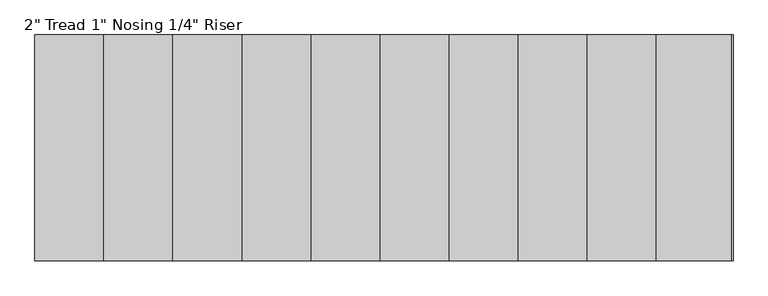
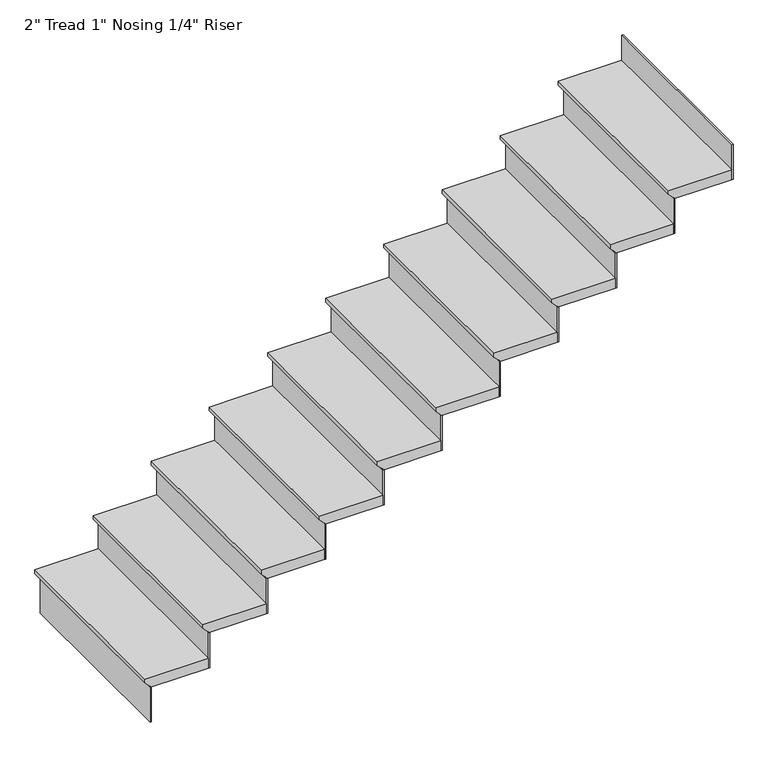
"""IFC4 building model written with IfcOpenShell, lengths in millimetres: stair flight geometry."""

from ifc_helpers import new_model, si_unit, frame, origin, place, context, project, spatial, polyline, outline, extrude, source, transform, mapped, element, save


def stair_flight_87f1d909(model_context):
    return source(origin(), model_context, "Body", "SweptSolid", [
        extrude(outline(polyline([(8432.8, -7947.6763529), (8432.8, -8252.4763529), (8413.75, -8252.4763529), (8388.35, -8227.0763529), (8382.0, -8227.0763529), (8382.0, -7947.6763529), (8432.8, -7947.6763529)])), frame((0.0, -3490.0338022, 0.0), z_axis=(0.0, 1.0, 0.0), x_axis=(0.0, 0.0, 1.0)), (0.0, 0.0, 1.0), 914.4),
        extrude(outline(polyline([(-8220.7263529, -3490.0338022), (-8227.0763529, -3490.0338022), (-8227.0763529, -2575.6338022), (-8220.7263529, -2575.6338022), (-8220.7263529, -3490.0338022)])), frame((0.0, 0.0, 8204.2), z_axis=(0.0, 0.0, 1.0), x_axis=(1.0, 0.0, 0.0)), (0.0, 0.0, 1.0), 177.8),
        extrude(outline(polyline([(-7941.3263529, -3490.0338022), (-7947.6763529, -3490.0338022), (-7947.6763529, -2575.6338022), (-7941.3263529, -2575.6338022), (-7941.3263529, -3490.0338022)])), frame((0.0, 0.0, 8382.0), z_axis=(0.0, 0.0, 1.0), x_axis=(1.0, 0.0, 0.0)), (0.0, 0.0, 1.0), 177.8),
        extrude(outline(polyline([(8610.6, -7668.2763529), (8610.6, -7973.0763529), (8591.55, -7973.0763529), (8566.15, -7947.6763529), (8559.8, -7947.6763529), (8559.8, -7668.2763529), (8610.6, -7668.2763529)])), frame((0.0, -3490.0338022, 0.0), z_axis=(0.0, 1.0, 0.0), x_axis=(0.0, 0.0, 1.0)), (0.0, 0.0, 1.0), 914.4),
        extrude(outline(polyline([(-7661.9263529, -3490.0338022), (-7668.2763529, -3490.0338022), (-7668.2763529, -2575.6338022), (-7661.9263529, -2575.6338022), (-7661.9263529, -3490.0338022)])), frame((0.0, 0.0, 8559.8), z_axis=(0.0, 0.0, 1.0), x_axis=(1.0, 0.0, 0.0)), (0.0, 0.0, 1.0), 177.8),
        extrude(outline(polyline([(8788.4, -7388.8763529), (8788.4, -7693.6763529), (8769.35, -7693.6763529), (8743.95, -7668.2763529), (8737.6, -7668.2763529), (8737.6, -7388.8763529), (8788.4, -7388.8763529)])), frame((0.0, -3490.0338022, 0.0), z_axis=(0.0, 1.0, 0.0), x_axis=(0.0, 0.0, 1.0)), (0.0, 0.0, 1.0), 914.4),
        extrude(outline(polyline([(-7382.5263529, -3490.0338022), (-7388.8763529, -3490.0338022), (-7388.8763529, -2575.6338022), (-7382.5263529, -2575.6338022), (-7382.5263529, -3490.0338022)])), frame((0.0, 0.0, 8737.6), z_axis=(0.0, 0.0, 1.0), x_axis=(1.0, 0.0, 0.0)), (0.0, 0.0, 1.0), 177.8),
        extrude(outline(polyline([(8966.2, -7109.4763529), (8966.2, -7414.2763529), (8947.15, -7414.2763529), (8921.75, -7388.8763529), (8915.4, -7388.8763529), (8915.4, -7109.4763529), (8966.2, -7109.4763529)])), frame((0.0, -3490.0338022, 0.0), z_axis=(0.0, 1.0, 0.0), x_axis=(0.0, 0.0, 1.0)), (0.0, 0.0, 1.0), 914.4),
        extrude(outline(polyline([(-7103.1263529, -3490.0338022), (-7109.4763529, -3490.0338022), (-7109.4763529, -2575.6338022), (-7103.1263529, -2575.6338022), (-7103.1263529, -3490.0338022)])), frame((0.0, 0.0, 8915.4), z_axis=(0.0, 0.0, 1.0), x_axis=(1.0, 0.0, 0.0)), (0.0, 0.0, 1.0), 177.8),
        extrude(outline(polyline([(9144.0, -6830.0763529), (9144.0, -7134.8763529), (9124.95, -7134.8763529), (9099.55, -7109.4763529), (9093.2, -7109.4763529), (9093.2, -6830.0763529), (9144.0, -6830.0763529)])), frame((0.0, -3490.0338022, 0.0), z_axis=(0.0, 1.0, 0.0), x_axis=(0.0, 0.0, 1.0)), (0.0, 0.0, 1.0), 914.4),
        extrude(outline(polyline([(-6823.7263529, -3490.0338022), (-6830.0763529, -3490.0338022), (-6830.0763529, -2575.6338022), (-6823.7263529, -2575.6338022), (-6823.7263529, -3490.0338022)])), frame((0.0, 0.0, 9093.2), z_axis=(0.0, 0.0, 1.0), x_axis=(1.0, 0.0, 0.0)), (0.0, 0.0, 1.0), 177.8),
        extrude(outline(polyline([(9321.8, -6550.6763529), (9321.8, -6855.4763529), (9302.75, -6855.4763529), (9277.35, -6830.0763529), (9271.0, -6830.0763529), (9271.0, -6550.6763529), (9321.8, -6550.6763529)])), frame((0.0, -3490.0338022, 0.0), z_axis=(0.0, 1.0, 0.0), x_axis=(0.0, 0.0, 1.0)), (0.0, 0.0, 1.0), 914.4),
        extrude(outline(polyline([(-6544.3263529, -3490.0338022), (-6550.6763529, -3490.0338022), (-6550.6763529, -2575.6338022), (-6544.3263529, -2575.6338022), (-6544.3263529, -3490.0338022)])), frame((0.0, 0.0, 9271.0), z_axis=(0.0, 0.0, 1.0), x_axis=(1.0, 0.0, 0.0)), (0.0, 0.0, 1.0), 177.8),
        extrude(outline(polyline([(9499.6, -6271.2763529), (9499.6, -6576.0763529), (9480.55, -6576.0763529), (9455.15, -6550.6763529), (9448.8, -6550.6763529), (9448.8, -6271.2763529), (9499.6, -6271.2763529)])), frame((0.0, -3490.0338022, 0.0), z_axis=(0.0, 1.0, 0.0), x_axis=(0.0, 0.0, 1.0)), (0.0, 0.0, 1.0), 914.4),
        extrude(outline(polyline([(-6264.9263529, -3490.0338022), (-6271.2763529, -3490.0338022), (-6271.2763529, -2575.6338022), (-6264.9263529, -2575.6338022), (-6264.9263529, -3490.0338022)])), frame((0.0, 0.0, 9448.8), z_axis=(0.0, 0.0, 1.0), x_axis=(1.0, 0.0, 0.0)), (0.0, 0.0, 1.0), 177.8),
        extrude(outline(polyline([(9677.4, -5991.8763529), (9677.4, -6296.6763529), (9658.35, -6296.6763529), (9632.95, -6271.2763529), (9626.6, -6271.2763529), (9626.6, -5991.8763529), (9677.4, -5991.8763529)])), frame((0.0, -3490.0338022, 0.0), z_axis=(0.0, 1.0, 0.0), x_axis=(0.0, 0.0, 1.0)), (0.0, 0.0, 1.0), 914.4),
        extrude(outline(polyline([(-5985.5263529, -3490.0338022), (-5991.8763529, -3490.0338022), (-5991.8763529, -2575.6338022), (-5985.5263529, -2575.6338022), (-5985.5263529, -3490.0338022)])), frame((0.0, 0.0, 9626.6), z_axis=(0.0, 0.0, 1.0), x_axis=(1.0, 0.0, 0.0)), (0.0, 0.0, 1.0), 177.8),
        extrude(outline(polyline([(9855.2, -5712.4763529), (9855.2, -6017.2763529), (9836.15, -6017.2763529), (9810.75, -5991.8763529), (9804.4, -5991.8763529), (9804.4, -5712.4763529), (9855.2, -5712.4763529)])), frame((0.0, -3490.0338022, 0.0), z_axis=(0.0, 1.0, 0.0), x_axis=(0.0, 0.0, 1.0)), (0.0, 0.0, 1.0), 914.4),
        extrude(outline(polyline([(-5706.1263529, -3490.0338022), (-5712.4763529, -3490.0338022), (-5712.4763529, -2575.6338022), (-5706.1263529, -2575.6338022), (-5706.1263529, -3490.0338022)])), frame((0.0, 0.0, 9804.4), z_axis=(0.0, 0.0, 1.0), x_axis=(1.0, 0.0, 0.0)), (0.0, 0.0, 1.0), 177.8),
        extrude(outline(polyline([(-5426.7263529, -3490.0338022), (-5433.0763529, -3490.0338022), (-5433.0763529, -2575.6338022), (-5426.7263529, -2575.6338022), (-5426.7263529, -3490.0338022)])), frame((0.0, 0.0, 9982.2), z_axis=(0.0, 0.0, 1.0), x_axis=(1.0, 0.0, 0.0)), (0.0, 0.0, 1.0), 177.8),
        extrude(outline(polyline([(10033.0, -5433.0763529), (10033.0, -5737.8763529), (10013.95, -5737.8763529), (9988.55, -5712.4763529), (9982.2, -5712.4763529), (9982.2, -5433.0763529), (10033.0, -5433.0763529)])), frame((0.0, -3490.0338022, 0.0), z_axis=(0.0, 1.0, 0.0), x_axis=(0.0, 0.0, 1.0)), (0.0, 0.0, 1.0), 914.4),
    ])


if __name__ == "__main__":
    model = new_model("IFC4")
    model_context = context("Model", 3, world=origin())
    ifc_project = project(units=[si_unit("LENGTHUNIT", "METRE", prefix="MILLI")], contexts=[model_context])
    site = spatial("IfcSite", under=ifc_project)
    building = spatial("IfcBuilding", under=site)
    placement = place(None, origin())
    stair_flight_shape = stair_flight_87f1d909(model_context)
    element("IfcStairFlight", 1, ObjectType="2\" Tread 1\" Nosing 1/4\" Riser", at=placement, inside=building, context=model_context, shape_type="MappedRepresentation", body=[
        mapped(stair_flight_shape, transform((0.0, 0.0, 0.0), x_axis=(1.0, 0.0, 0.0), y_axis=(0.0, 1.0, 0.0), z_axis=(0.0, 0.0, 1.0))),
    ])
    save(model, "model.ifc")
